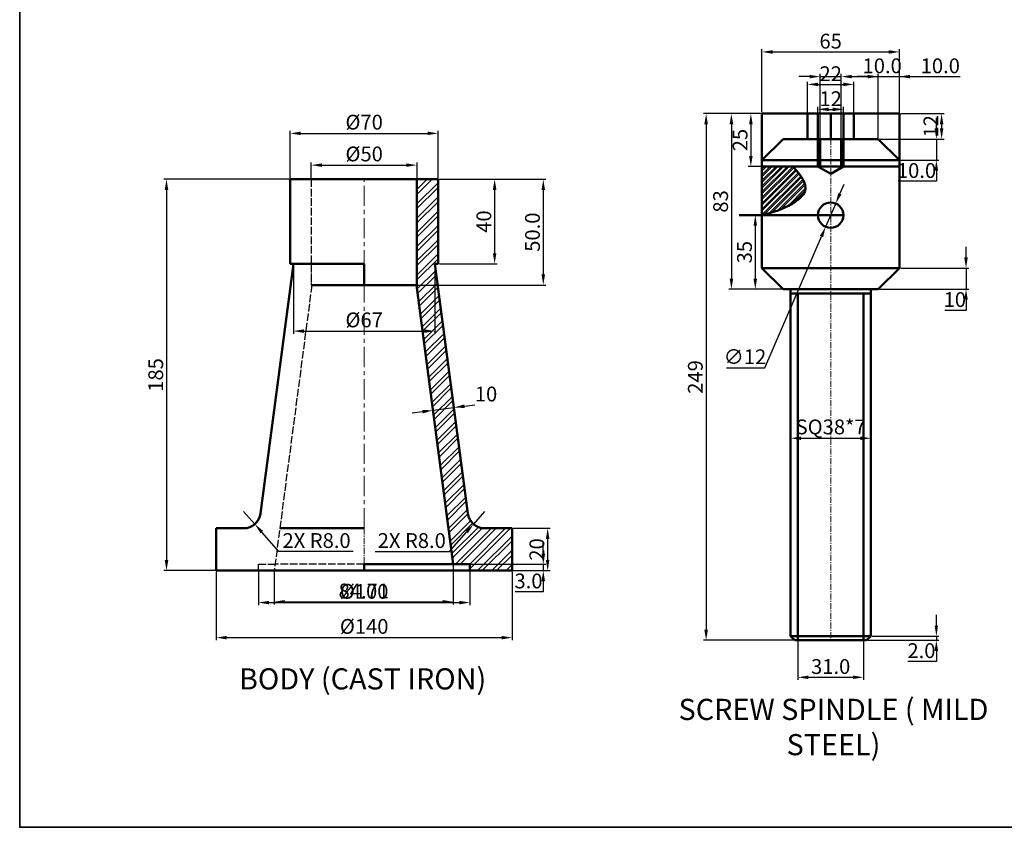
# Model space of a CAD drawing. Units: millimetres. Extents: x 4274 to 5106, y 2129 to 2785.
# Tile 1 of 4: x 4274 to 4740, y 2140 to 2522. Entities that reach past the tile are written whole.
import ezdxf

# ---------------------------------------------------------------- set-up
doc = ezdxf.new("R2010")
doc.units = ezdxf.units.MM
doc.header["$LTSCALE"] = 0.3
doc.linetypes.add('ACAD_ISO02W100', pattern=[15, 12, -3])
doc.linetypes.add('CENTER', pattern=[50.8, 31.75, -6.35, 6.35, -6.35])
for name, color, linetype, lineweight in [('M-CNTR', 1, 'CENTER', 18), ('M-DIMS', 2, 'Continuous', 25), ('M-HATC', 8, 'Continuous', 18), ('M-HIDN', 8, 'ACAD_ISO02W100', 25), ('M-OUTL', 7, 'Continuous', 50), ('M-TEXT', 3, 'Continuous', 25), ('M-TTLB', 7, 'Continuous', 35)]:
    doc.layers.add(name, color=color, linetype=linetype, lineweight=lineweight)
doc.styles.get("Standard").update_dxf_attribs({"font": 'arial.ttf'})
doc.dimstyles.new('ISO-25', dxfattribs={"dimtxt": 7, "dimasz": 5, "dimexe": 1.25, "dimexo": 0.625, "dimtad": 1, "dimtoh": 1, "dimtxsty": 'Standard', "dimcen": 2.5, "dimadec": 0, "dimazin": 0, "dimtfac": 1, "dimtmove": 0, "dimatfit": 3, "dimfxl": 1, "dimarcsym": 0})

# ---------------------------------------------------------------- blocks, each defined once
blk = doc.blocks.new('*D1')
at = {"layer": 'Defpoints', "color": 0, "ltscale": 0.3, "transparency": 16777216}
for p in [(4366.95, 2261.27), (4506.95, 2261.27), (4506.95, 2229.58)]:
    blk.add_point(p, dxfattribs=at)
at = {"layer": 'M-DIMS', "color": 0, "lineweight": -2, "ltscale": 0.3, "transparency": 16777216}
for p, q in [((4366.95, 2260.64), (4366.95, 2228.33)), ((4506.95, 2260.64), (4506.95, 2228.33)), ((4371.95, 2229.58), (4501.95, 2229.58))]:
    blk.add_line(p, q, dxfattribs=at)
at = {"layer": 'M-DIMS', "color": 0, "ltscale": 0.3, "transparency": 16777216}
for points in [[(4371.95, 2230.41), (4371.95, 2228.74), (4366.95, 2229.58)], [(4501.95, 2230.41), (4501.95, 2228.74), (4506.95, 2229.58)]]:
    blk.add_solid(points, dxfattribs=at)
at = {"layer": 'M-DIMS', "color": 0, "ltscale": 0.3, "transparency": 16777216, "insert": (4436.95, 2233.97), "char_height": 7, "attachment_point": 5}
blk.add_mtext('%%C140', dxfattribs=at)
blk = doc.blocks.new('*D2')
at = {"layer": 'Defpoints', "color": 0, "ltscale": 0.3, "transparency": 16777216}
for p in [(4386.95, 2261.27), (4486.95, 2261.27), (4486.95, 2246.14)]:
    blk.add_point(p, dxfattribs=at)
at = {"layer": 'M-DIMS', "color": 0, "lineweight": -2, "ltscale": 0.3, "transparency": 16777216}
for p, q in [((4386.95, 2260.64), (4386.95, 2244.89)), ((4486.95, 2260.64), (4486.95, 2244.89)), ((4391.95, 2246.14), (4481.95, 2246.14))]:
    blk.add_line(p, q, dxfattribs=at)
at = {"layer": 'M-DIMS', "color": 0, "ltscale": 0.3, "transparency": 16777216}
for points in [[(4391.95, 2246.98), (4391.95, 2245.31), (4386.95, 2246.14)], [(4481.95, 2246.98), (4481.95, 2245.31), (4486.95, 2246.14)]]:
    blk.add_solid(points, dxfattribs=at)
at = {"layer": 'M-DIMS', "color": 0, "ltscale": 0.3, "transparency": 16777216, "insert": (4436.95, 2250.54), "char_height": 7, "attachment_point": 5}
blk.add_mtext('%%C100', dxfattribs=at)
blk = doc.blocks.new('*D3')
at = {"layer": 'Defpoints', "color": 0, "ltscale": 0.3, "transparency": 16777216}
for p in [(4506.95, 2281.27), (4506.95, 2261.27), (4523.77, 2261.27)]:
    blk.add_point(p, dxfattribs=at)
at = {"layer": 'M-DIMS', "color": 0, "lineweight": -2, "ltscale": 0.3, "transparency": 16777216}
for p, q in [((4507.57, 2281.27), (4525.02, 2281.27)), ((4523.77, 2276.27), (4523.77, 2266.27)), ((4507.57, 2261.27), (4525.02, 2261.27))]:
    blk.add_line(p, q, dxfattribs=at)
at = {"layer": 'M-DIMS', "color": 0, "ltscale": 0.3, "transparency": 16777216}
for points in [[(4522.93, 2276.27), (4524.6, 2276.27), (4523.77, 2281.27)], [(4522.93, 2266.27), (4524.6, 2266.27), (4523.77, 2261.27)]]:
    blk.add_solid(points, dxfattribs=at)
at = {"layer": 'M-DIMS', "color": 0, "ltscale": 0.3, "transparency": 16777216, "insert": (4519.57, 2271.27), "char_height": 7, "attachment_point": 5, "rotation": 90}
blk.add_mtext('20', dxfattribs=at)
blk = doc.blocks.new('*D4')
at = {"layer": 'Defpoints', "color": 0, "ltscale": 0.3, "transparency": 16777216}
for p in [(4436.95, 2446.27), (4343.43, 2261.27), (4436.95, 2261.27)]:
    blk.add_point(p, dxfattribs=at)
at = {"layer": 'M-DIMS', "color": 0, "lineweight": -2, "ltscale": 0.3, "transparency": 16777216}
for p, q in [((4436.32, 2446.27), (4342.18, 2446.27)), ((4343.43, 2441.27), (4343.43, 2266.27)), ((4436.32, 2261.27), (4342.18, 2261.27))]:
    blk.add_line(p, q, dxfattribs=at)
at = {"layer": 'M-DIMS', "color": 0, "ltscale": 0.3, "transparency": 16777216}
for points in [[(4342.6, 2441.27), (4344.27, 2441.27), (4343.43, 2446.27)], [(4342.6, 2266.27), (4344.27, 2266.27), (4343.43, 2261.27)]]:
    blk.add_solid(points, dxfattribs=at)
at = {"layer": 'M-DIMS', "color": 0, "ltscale": 0.3, "transparency": 16777216, "insert": (4339.23, 2353.77), "char_height": 7, "attachment_point": 5, "rotation": 90}
blk.add_mtext('185', dxfattribs=at)
blk = doc.blocks.new('*D5')
at = {"layer": 'Defpoints', "color": 0, "ltscale": 0.3, "transparency": 16777216}
for p in [(4471.95, 2446.27), (4471.95, 2406.27), (4498.68, 2406.27)]:
    blk.add_point(p, dxfattribs=at)
at = {"layer": 'M-DIMS', "color": 0, "lineweight": -2, "ltscale": 0.3, "transparency": 16777216}
for p, q in [((4472.57, 2446.27), (4499.93, 2446.27)), ((4498.68, 2441.27), (4498.68, 2411.27)), ((4472.57, 2406.27), (4499.93, 2406.27))]:
    blk.add_line(p, q, dxfattribs=at)
at = {"layer": 'M-DIMS', "color": 0, "ltscale": 0.3, "transparency": 16777216}
for points in [[(4497.85, 2441.27), (4499.52, 2441.27), (4498.68, 2446.27)], [(4497.85, 2411.27), (4499.52, 2411.27), (4498.68, 2406.27)]]:
    blk.add_solid(points, dxfattribs=at)
at = {"layer": 'M-DIMS', "color": 0, "ltscale": 0.3, "transparency": 16777216, "insert": (4494.48, 2426.27), "char_height": 7, "attachment_point": 5, "rotation": 90}
blk.add_mtext('40', dxfattribs=at)
blk = doc.blocks.new('*D6')
at = {"layer": 'Defpoints', "color": 0, "ltscale": 0.3, "transparency": 16777216}
for p in [(4471.95, 2467.97), (4401.95, 2446.27), (4471.95, 2446.27)]:
    blk.add_point(p, dxfattribs=at)
at = {"layer": 'M-DIMS', "color": 0, "lineweight": -2, "ltscale": 0.3, "transparency": 16777216}
for p, q in [((4401.95, 2446.89), (4401.95, 2469.22)), ((4471.95, 2446.89), (4471.95, 2469.22)), ((4406.95, 2467.97), (4466.95, 2467.97))]:
    blk.add_line(p, q, dxfattribs=at)
at = {"layer": 'M-DIMS', "color": 0, "ltscale": 0.3, "transparency": 16777216}
for points in [[(4406.95, 2468.81), (4406.95, 2467.14), (4401.95, 2467.97)], [(4466.95, 2468.81), (4466.95, 2467.14), (4471.95, 2467.97)]]:
    blk.add_solid(points, dxfattribs=at)
at = {"layer": 'M-DIMS', "color": 0, "ltscale": 0.3, "transparency": 16777216, "insert": (4436.95, 2472.37), "char_height": 7, "attachment_point": 5}
blk.add_mtext('%%C70', dxfattribs=at)
blk = doc.blocks.new('*D7')
at = {"layer": 'Defpoints', "color": 0, "ltscale": 0.3, "transparency": 16777216}
for p in [(4461.95, 2452.96), (4411.95, 2446.27), (4461.95, 2446.27)]:
    blk.add_point(p, dxfattribs=at)
at = {"layer": 'M-DIMS', "color": 0, "lineweight": -2, "ltscale": 0.3, "transparency": 16777216}
for p, q in [((4411.95, 2446.89), (4411.95, 2454.21)), ((4416.95, 2452.96), (4456.95, 2452.96)), ((4461.95, 2446.89), (4461.95, 2454.21))]:
    blk.add_line(p, q, dxfattribs=at)
at = {"layer": 'M-DIMS', "color": 0, "ltscale": 0.3, "transparency": 16777216}
for points in [[(4416.95, 2453.79), (4416.95, 2452.13), (4411.95, 2452.96)], [(4456.95, 2453.79), (4456.95, 2452.13), (4461.95, 2452.96)]]:
    blk.add_solid(points, dxfattribs=at)
at = {"layer": 'M-DIMS', "color": 0, "ltscale": 0.3, "transparency": 16777216, "insert": (4436.95, 2457.35), "char_height": 7, "attachment_point": 5}
blk.add_mtext('%%C50', dxfattribs=at)
blk = doc.blocks.new('*D8')
at = {"layer": 'Defpoints', "color": 0, "ltscale": 0.3, "transparency": 16777216}
for p in [(4403.45, 2406.27), (4470.45, 2406.27), (4470.45, 2374.49)]:
    blk.add_point(p, dxfattribs=at)
at = {"layer": 'M-DIMS', "color": 0, "lineweight": -2, "ltscale": 0.3, "transparency": 16777216}
for p, q in [((4403.45, 2405.64), (4403.45, 2373.24)), ((4470.45, 2405.64), (4470.45, 2373.24)), ((4408.45, 2374.49), (4465.45, 2374.49))]:
    blk.add_line(p, q, dxfattribs=at)
at = {"layer": 'M-DIMS', "color": 0, "ltscale": 0.3, "transparency": 16777216}
for points in [[(4408.45, 2375.33), (4408.45, 2373.66), (4403.45, 2374.49)], [(4465.45, 2375.33), (4465.45, 2373.66), (4470.45, 2374.49)]]:
    blk.add_solid(points, dxfattribs=at)
at = {"layer": 'M-DIMS', "color": 0, "ltscale": 0.3, "transparency": 16777216, "insert": (4436.95, 2378.89), "char_height": 7, "attachment_point": 5}
blk.add_mtext('%%C67', dxfattribs=at)
blk = doc.blocks.new('*D9')
at = {"layer": 'Defpoints', "color": 0, "ltscale": 0.3, "transparency": 16777216}
for p in [(4469.5, 2337.04), (4479.41, 2338.34), (4479.41, 2338.34)]:
    blk.add_point(p, dxfattribs=at)
at = {"layer": 'M-DIMS', "color": 0, "lineweight": -2, "ltscale": 0.3, "transparency": 16777216}
for p, q in [((4479.33, 2338.96), (4479.25, 2339.58)), ((4484.37, 2339), (4489.33, 2339.65)), ((4464.54, 2336.38), (4459.59, 2335.73)), ((4469.42, 2337.66), (4469.34, 2338.28)), ((4469.5, 2337.04), (4479.41, 2338.34))]:
    blk.add_line(p, q, dxfattribs=at)
at = {"layer": 'M-DIMS', "color": 0, "ltscale": 0.3, "transparency": 16777216}
for points in [[(4484.26, 2339.83), (4484.48, 2338.17), (4479.41, 2338.34)], [(4464.43, 2337.21), (4464.65, 2335.56), (4469.5, 2337.04)]]:
    blk.add_solid(points, dxfattribs=at)
at = {"layer": 'M-DIMS', "color": 0, "ltscale": 0.3, "transparency": 16777216, "insert": (4494.62, 2343.85), "char_height": 7, "attachment_point": 5}
blk.add_mtext('10', dxfattribs=at)
blk = doc.blocks.new('*D42')
at = {"layer": 'Defpoints', "color": 0, "ltscale": 0.3, "transparency": 16777216}
for p in [(4663.68, 2479.33), (4651.68, 2477.31), (4663.68, 2477.31)]:
    blk.add_point(p, dxfattribs=at)
at = {"layer": 'M-DIMS', "color": 0, "lineweight": -2, "ltscale": 0.3, "transparency": 16777216}
for p, q in [((4651.68, 2477.94), (4651.68, 2480.58)), ((4656.68, 2479.33), (4658.68, 2479.33)), ((4663.68, 2477.94), (4663.68, 2480.58))]:
    blk.add_line(p, q, dxfattribs=at)
at = {"layer": 'M-DIMS', "color": 0, "ltscale": 0.3, "transparency": 16777216}
for points in [[(4656.68, 2480.17), (4656.68, 2478.5), (4651.68, 2479.33)], [(4658.68, 2480.17), (4658.68, 2478.5), (4663.68, 2479.33)]]:
    blk.add_solid(points, dxfattribs=at)
at = {"layer": 'M-DIMS', "color": 0, "ltscale": 0.3, "transparency": 16777216, "insert": (4657.68, 2483.47), "char_height": 7, "attachment_point": 5}
blk.add_mtext('12', dxfattribs=at)
blk = doc.blocks.new('*D43')
at = {"layer": 'Defpoints', "color": 0, "ltscale": 0.3, "transparency": 16777216}
for p in [(4668.68, 2491.13), (4646.68, 2477.31), (4668.68, 2477.31)]:
    blk.add_point(p, dxfattribs=at)
at = {"layer": 'M-DIMS', "color": 0, "lineweight": -2, "ltscale": 0.3, "transparency": 16777216}
for p, q in [((4646.68, 2477.94), (4646.68, 2492.38)), ((4651.68, 2491.13), (4663.68, 2491.13)), ((4668.68, 2477.94), (4668.68, 2492.38))]:
    blk.add_line(p, q, dxfattribs=at)
at = {"layer": 'M-DIMS', "color": 0, "ltscale": 0.3, "transparency": 16777216}
for points in [[(4651.68, 2491.96), (4651.68, 2490.29), (4646.68, 2491.13)], [(4663.68, 2491.96), (4663.68, 2490.29), (4668.68, 2491.13)]]:
    blk.add_solid(points, dxfattribs=at)
at = {"layer": 'M-DIMS', "color": 0, "ltscale": 0.3, "transparency": 16777216, "insert": (4657.68, 2495.27), "char_height": 7, "attachment_point": 5}
blk.add_mtext('22', dxfattribs=at)
blk = doc.blocks.new('*D44')
at = {"layer": 'Defpoints', "color": 0, "ltscale": 0.3, "transparency": 16777216}
for p in [(4690.18, 2506.47), (4625.18, 2477.31), (4690.18, 2477.31)]:
    blk.add_point(p, dxfattribs=at)
at = {"layer": 'M-DIMS', "color": 0, "lineweight": -2, "ltscale": 0.3, "transparency": 16777216}
for p, q in [((4625.18, 2477.94), (4625.18, 2507.72)), ((4630.18, 2506.47), (4685.18, 2506.47)), ((4690.18, 2477.94), (4690.18, 2507.72))]:
    blk.add_line(p, q, dxfattribs=at)
at = {"layer": 'M-DIMS', "color": 0, "ltscale": 0.3, "transparency": 16777216}
for points in [[(4630.18, 2507.3), (4630.18, 2505.64), (4625.18, 2506.47)], [(4685.18, 2507.3), (4685.18, 2505.64), (4690.18, 2506.47)]]:
    blk.add_solid(points, dxfattribs=at)
at = {"layer": 'M-DIMS', "color": 0, "ltscale": 0.3, "transparency": 16777216, "insert": (4657.68, 2510.67), "char_height": 7, "attachment_point": 5}
blk.add_mtext('65', dxfattribs=at)
blk = doc.blocks.new('*D45')
at = {"layer": 'Defpoints', "color": 0, "ltscale": 0.3, "transparency": 16777216}
for p in [(4690.18, 2477.31), (4680.18, 2465.31), (4710.16, 2465.31)]:
    blk.add_point(p, dxfattribs=at)
at = {"layer": 'M-DIMS', "color": 0, "lineweight": -2, "ltscale": 0.3, "transparency": 16777216}
for p, q in [((4690.8, 2477.31), (4711.41, 2477.31)), ((4710.16, 2472.31), (4710.16, 2470.31)), ((4680.8, 2465.31), (4711.41, 2465.31))]:
    blk.add_line(p, q, dxfattribs=at)
at = {"layer": 'M-DIMS', "color": 0, "ltscale": 0.3, "transparency": 16777216}
for points in [[(4709.33, 2472.31), (4710.99, 2472.31), (4710.16, 2477.31)], [(4709.33, 2470.31), (4710.99, 2470.31), (4710.16, 2465.31)]]:
    blk.add_solid(points, dxfattribs=at)
at = {"layer": 'M-DIMS', "color": 0, "ltscale": 0.3, "transparency": 16777216, "insert": (4706.02, 2471.31), "char_height": 7, "attachment_point": 5, "rotation": 90}
blk.add_mtext('12', dxfattribs=at)
blk = doc.blocks.new('*D46')
at = {"layer": 'Defpoints', "color": 0, "ltscale": 0.3, "transparency": 16777216}
for p in [(4690.18, 2404.31), (4680.18, 2394.31), (4721.72, 2394.31)]:
    blk.add_point(p, dxfattribs=at)
at = {"layer": 'M-DIMS', "color": 0, "lineweight": -2, "ltscale": 0.3, "transparency": 16777216}
for p, q in [((4721.72, 2409.31), (4721.72, 2414.31)), ((4690.8, 2404.31), (4722.97, 2404.31)), ((4721.72, 2404.31), (4721.72, 2394.31)), ((4680.8, 2394.31), (4722.97, 2394.31)), ((4721.72, 2389.31), (4721.72, 2384.31)), ((4721.72, 2384.31), (4711.75, 2384.31))]:
    blk.add_line(p, q, dxfattribs=at)
at = {"layer": 'M-DIMS', "color": 0, "ltscale": 0.3, "transparency": 16777216}
for points in [[(4720.88, 2409.31), (4722.55, 2409.31), (4721.72, 2404.31)], [(4720.88, 2389.31), (4722.55, 2389.31), (4721.72, 2394.31)]]:
    blk.add_solid(points, dxfattribs=at)
at = {"layer": 'M-DIMS', "color": 0, "ltscale": 0.3, "transparency": 16777216, "insert": (4716.42, 2388.51), "char_height": 7, "attachment_point": 5}
blk.add_mtext('10', dxfattribs=at)
blk = doc.blocks.new('*D47')
at = {"layer": 'Defpoints', "color": 0, "ltscale": 0.3, "transparency": 16777216}
for p in [(4625.18, 2477.31), (4598.74, 2228.31), (4640.68, 2228.31)]:
    blk.add_point(p, dxfattribs=at)
at = {"layer": 'M-DIMS', "color": 0, "lineweight": -2, "ltscale": 0.3, "transparency": 16777216}
for p, q in [((4624.55, 2477.31), (4597.49, 2477.31)), ((4598.74, 2472.31), (4598.74, 2233.31)), ((4640.05, 2228.31), (4597.49, 2228.31))]:
    blk.add_line(p, q, dxfattribs=at)
at = {"layer": 'M-DIMS', "color": 0, "ltscale": 0.3, "transparency": 16777216}
for points in [[(4597.91, 2472.31), (4599.57, 2472.31), (4598.74, 2477.31)], [(4597.91, 2233.31), (4599.57, 2233.31), (4598.74, 2228.31)]]:
    blk.add_solid(points, dxfattribs=at)
at = {"layer": 'M-DIMS', "color": 0, "ltscale": 0.3, "transparency": 16777216, "insert": (4594.54, 2352.81), "char_height": 7, "attachment_point": 5, "rotation": 90}
blk.add_mtext('249', dxfattribs=at)
blk = doc.blocks.new('*D48')
at = {"layer": 'Defpoints', "color": 0, "ltscale": 0.3, "transparency": 16777216}
for p in [(4625.18, 2477.31), (4610.71, 2394.31), (4635.18, 2394.31)]:
    blk.add_point(p, dxfattribs=at)
at = {"layer": 'M-DIMS', "color": 0, "lineweight": -2, "ltscale": 0.3, "transparency": 16777216}
for p, q in [((4624.55, 2477.31), (4609.46, 2477.31)), ((4610.71, 2472.31), (4610.71, 2399.31)), ((4634.55, 2394.31), (4609.46, 2394.31))]:
    blk.add_line(p, q, dxfattribs=at)
at = {"layer": 'M-DIMS', "color": 0, "ltscale": 0.3, "transparency": 16777216}
for points in [[(4609.88, 2472.31), (4611.55, 2472.31), (4610.71, 2477.31)], [(4609.88, 2399.31), (4611.55, 2399.31), (4610.71, 2394.31)]]:
    blk.add_solid(points, dxfattribs=at)
at = {"layer": 'M-DIMS', "color": 0, "ltscale": 0.3, "transparency": 16777216, "insert": (4606.51, 2435.81), "char_height": 7, "attachment_point": 5, "rotation": 90}
blk.add_mtext('83', dxfattribs=at)
blk = doc.blocks.new('*D49')
at = {"layer": 'Defpoints', "color": 0, "ltscale": 0.3, "transparency": 16777216}
for p in [(4625.18, 2429.31), (4622.01, 2394.31), (4635.18, 2394.31)]:
    blk.add_point(p, dxfattribs=at)
at = {"layer": 'M-DIMS', "color": 0, "lineweight": -2, "ltscale": 0.3, "transparency": 16777216}
for p, q in [((4624.55, 2429.31), (4620.76, 2429.31)), ((4622.01, 2424.31), (4622.01, 2399.31)), ((4634.55, 2394.31), (4620.76, 2394.31))]:
    blk.add_line(p, q, dxfattribs=at)
at = {"layer": 'M-DIMS', "color": 0, "ltscale": 0.3, "transparency": 16777216}
for points in [[(4621.17, 2424.31), (4622.84, 2424.31), (4622.01, 2429.31)], [(4621.17, 2399.31), (4622.84, 2399.31), (4622.01, 2394.31)]]:
    blk.add_solid(points, dxfattribs=at)
at = {"layer": 'M-DIMS', "color": 0, "ltscale": 0.3, "transparency": 16777216, "insert": (4617.81, 2411.81), "char_height": 7, "attachment_point": 5, "rotation": 90}
blk.add_mtext('35', dxfattribs=at)
blk = doc.blocks.new('*D50')
at = {"layer": 'Defpoints', "color": 0, "ltscale": 0.3, "transparency": 16777216}
for p in [(4625.18, 2477.31), (4619.92, 2452.31), (4625.18, 2452.31)]:
    blk.add_point(p, dxfattribs=at)
at = {"layer": 'M-DIMS', "color": 0, "lineweight": -2, "ltscale": 0.3, "transparency": 16777216}
for p, q in [((4624.55, 2477.31), (4618.67, 2477.31)), ((4619.92, 2472.31), (4619.92, 2457.31)), ((4624.55, 2452.31), (4618.67, 2452.31))]:
    blk.add_line(p, q, dxfattribs=at)
at = {"layer": 'M-DIMS', "color": 0, "ltscale": 0.3, "transparency": 16777216}
for points in [[(4619.09, 2472.31), (4620.75, 2472.31), (4619.92, 2477.31)], [(4619.09, 2457.31), (4620.75, 2457.31), (4619.92, 2452.31)]]:
    blk.add_solid(points, dxfattribs=at)
at = {"layer": 'M-DIMS', "color": 0, "ltscale": 0.3, "transparency": 16777216, "insert": (4615.72, 2464.81), "char_height": 7, "attachment_point": 5, "rotation": 90}
blk.add_mtext('25', dxfattribs=at)
blk = doc.blocks.new('*D51')
at = {"layer": 'Defpoints', "color": 0, "ltscale": 0.3, "transparency": 16777216}
for p in [(4676.68, 2323.83), (4638.68, 2312.31), (4676.68, 2312.31)]:
    blk.add_point(p, dxfattribs=at)
at = {"layer": 'M-DIMS', "color": 0, "lineweight": -2, "ltscale": 0.3, "transparency": 16777216}
for p, q in [((4638.68, 2312.94), (4638.68, 2325.08)), ((4676.68, 2312.94), (4676.68, 2325.08)), ((4643.68, 2323.83), (4671.68, 2323.83))]:
    blk.add_line(p, q, dxfattribs=at)
at = {"layer": 'M-DIMS', "color": 0, "ltscale": 0.3, "transparency": 16777216}
for points in [[(4643.68, 2324.66), (4643.68, 2323), (4638.68, 2323.83)], [(4671.68, 2324.66), (4671.68, 2323), (4676.68, 2323.83)]]:
    blk.add_solid(points, dxfattribs=at)
at = {"layer": 'M-DIMS', "color": 0, "ltscale": 0.3, "transparency": 16777216, "insert": (4657.68, 2328.29), "char_height": 7, "attachment_point": 5}
blk.add_mtext('SQ38*7', dxfattribs=at)
blk = doc.blocks.new('*D52')
at = {"layer": 'Defpoints', "color": 0, "ltscale": 0.3, "transparency": 16777216}
for p in [(4660.05, 2434.82), (4655.3, 2423.8)]:
    blk.add_point(p, dxfattribs=at)
at = {"layer": 'M-DIMS', "color": 0, "lineweight": -2, "ltscale": 0.3, "transparency": 16777216}
for p, q in [((4662.03, 2439.41), (4664.01, 2444.01)), ((4660.05, 2434.82), (4655.3, 2423.8)), ((4626.53, 2357.07), (4653.32, 2419.21)), ((4608.33, 2357.07), (4626.53, 2357.07))]:
    blk.add_line(p, q, dxfattribs=at)
at = {"layer": 'M-DIMS', "color": 0, "ltscale": 0.3, "transparency": 16777216}
for points in [[(4661.27, 2439.74), (4662.8, 2439.08), (4660.05, 2434.82)], [(4652.56, 2419.54), (4654.09, 2418.88), (4655.3, 2423.8)]]:
    blk.add_solid(points, dxfattribs=at)
at = {"layer": 'M-DIMS', "color": 0, "ltscale": 0.3, "transparency": 16777216, "insert": (4617.12, 2361.46), "char_height": 7, "attachment_point": 5}
blk.add_mtext('∅12', dxfattribs=at)
blk = doc.blocks.new('*D62')
at = {"layer": 'Defpoints', "color": 0, "ltscale": 0.3, "transparency": 16777216}
for p in [(4461.95, 2446.27), (4461.68, 2396.27), (4521.7, 2396.27)]:
    blk.add_point(p, dxfattribs=at)
at = {"layer": 'M-DIMS', "color": 0, "lineweight": -2, "ltscale": 0.3, "transparency": 16777216}
for p, q in [((4462.57, 2446.27), (4522.95, 2446.27)), ((4521.7, 2441.27), (4521.7, 2401.27)), ((4462.31, 2396.27), (4522.95, 2396.27))]:
    blk.add_line(p, q, dxfattribs=at)
at = {"layer": 'M-DIMS', "color": 0, "ltscale": 0.3, "transparency": 16777216}
for points in [[(4520.86, 2441.27), (4522.53, 2441.27), (4521.7, 2446.27)], [(4520.86, 2401.27), (4522.53, 2401.27), (4521.7, 2396.27)]]:
    blk.add_solid(points, dxfattribs=at)
at = {"layer": 'M-DIMS', "color": 0, "ltscale": 0.3, "transparency": 16777216, "insert": (4517.5, 2421.27), "char_height": 7, "attachment_point": 5, "rotation": 90}
blk.add_mtext('50.0', dxfattribs=at)
blk = doc.blocks.new('*D63')
at = {"layer": 'Defpoints', "color": 0, "ltscale": 0.3, "transparency": 16777216}
for p in [(4479.1, 2264.27), (4394.39, 2261.27), (4479.1, 2246.52)]:
    blk.add_point(p, dxfattribs=at)
at = {"layer": 'M-DIMS', "color": 0, "lineweight": -2, "ltscale": 0.3, "transparency": 16777216}
for p, q in [((4394.39, 2260.64), (4394.39, 2245.27)), ((4479.1, 2263.64), (4479.1, 2245.27)), ((4399.39, 2246.52), (4474.1, 2246.52))]:
    blk.add_line(p, q, dxfattribs=at)
at = {"layer": 'M-DIMS', "color": 0, "ltscale": 0.3, "transparency": 16777216}
for points in [[(4399.39, 2247.35), (4399.39, 2245.68), (4394.39, 2246.52)], [(4474.1, 2247.35), (4474.1, 2245.68), (4479.1, 2246.52)]]:
    blk.add_solid(points, dxfattribs=at)
at = {"layer": 'M-DIMS', "color": 0, "ltscale": 0.3, "transparency": 16777216, "insert": (4436.75, 2250.72), "char_height": 7, "attachment_point": 5}
blk.add_mtext('84.71', dxfattribs=at)
blk = doc.blocks.new('*D64')
at = {"layer": 'Defpoints', "color": 0, "ltscale": 0.3, "transparency": 16777216}
for p in [(4486.95, 2264.27), (4486.95, 2261.27), (4521.7, 2261.27)]:
    blk.add_point(p, dxfattribs=at)
at = {"layer": 'M-DIMS', "color": 0, "lineweight": -2, "ltscale": 0.3, "transparency": 16777216}
for p, q in [((4521.7, 2269.27), (4521.7, 2274.27)), ((4487.57, 2264.27), (4522.95, 2264.27)), ((4521.7, 2264.27), (4521.7, 2261.27)), ((4487.57, 2261.27), (4522.95, 2261.27)), ((4521.7, 2256.27), (4521.7, 2251.27)), ((4521.7, 2251.27), (4508.36, 2251.27))]:
    blk.add_line(p, q, dxfattribs=at)
at = {"layer": 'M-DIMS', "color": 0, "ltscale": 0.3, "transparency": 16777216}
for points in [[(4520.86, 2269.27), (4522.53, 2269.27), (4521.7, 2264.27)], [(4520.86, 2256.27), (4522.53, 2256.27), (4521.7, 2261.27)]]:
    blk.add_solid(points, dxfattribs=at)
at = {"layer": 'M-DIMS', "color": 0, "ltscale": 0.3, "transparency": 16777216, "insert": (4514.71, 2255.47), "char_height": 7, "attachment_point": 5}
blk.add_mtext('3.0', dxfattribs=at)
blk = doc.blocks.new('*D65')
at = {"layer": 'Defpoints', "color": 0, "ltscale": 0.3, "transparency": 16777216}
for p in [(4680.18, 2465.31), (4690.18, 2455.31), (4707.68, 2455.31)]:
    blk.add_point(p, dxfattribs=at)
at = {"layer": 'M-DIMS', "color": 0, "lineweight": -2, "ltscale": 0.3, "transparency": 16777216}
for p, q in [((4707.68, 2470.31), (4707.68, 2475.31)), ((4680.8, 2465.31), (4708.93, 2465.31)), ((4707.68, 2465.31), (4707.68, 2455.31)), ((4690.8, 2455.31), (4708.93, 2455.31)), ((4707.68, 2450.31), (4707.68, 2445.31)), ((4707.68, 2445.31), (4689.55, 2445.31))]:
    blk.add_line(p, q, dxfattribs=at)
at = {"layer": 'M-DIMS', "color": 0, "ltscale": 0.3, "transparency": 16777216}
for points in [[(4706.84, 2470.31), (4708.51, 2470.31), (4707.68, 2465.31)], [(4706.84, 2450.31), (4708.51, 2450.31), (4707.68, 2455.31)]]:
    blk.add_solid(points, dxfattribs=at)
at = {"layer": 'M-DIMS', "color": 0, "ltscale": 0.3, "transparency": 16777216, "insert": (4698.3, 2449.51), "char_height": 7, "attachment_point": 5}
blk.add_mtext('10.0', dxfattribs=at)
blk = doc.blocks.new('*D66')
at = {"layer": 'Defpoints', "color": 0, "ltscale": 0.3, "transparency": 16777216}
for p in [(4690.18, 2494.81), (4680.18, 2465.31), (4690.18, 2455.31)]:
    blk.add_point(p, dxfattribs=at)
at = {"layer": 'M-DIMS', "color": 0, "lineweight": -2, "ltscale": 0.3, "transparency": 16777216}
for p, q in [((4675.18, 2494.81), (4670.18, 2494.81)), ((4680.18, 2465.94), (4680.18, 2496.06)), ((4680.18, 2494.81), (4690.18, 2494.81)), ((4690.18, 2455.94), (4690.18, 2496.06)), ((4695.18, 2494.81), (4718.93, 2494.81))]:
    blk.add_line(p, q, dxfattribs=at)
at = {"layer": 'M-DIMS', "color": 0, "ltscale": 0.3, "transparency": 16777216}
for points in [[(4675.18, 2495.65), (4675.18, 2493.98), (4680.18, 2494.81)], [(4695.18, 2495.65), (4695.18, 2493.98), (4690.18, 2494.81)]]:
    blk.add_solid(points, dxfattribs=at)
at = {"layer": 'M-DIMS', "color": 0, "ltscale": 0.3, "transparency": 16777216, "insert": (4709.55, 2499.01), "char_height": 7, "attachment_point": 5}
blk.add_mtext('10.0', dxfattribs=at)
blk = doc.blocks.new('*D67')
at = {"layer": 'Defpoints', "color": 0, "ltscale": 0.3, "transparency": 16777216}
for p in [(4662.68, 2494.81), (4652.68, 2465.31), (4662.68, 2465.31)]:
    blk.add_point(p, dxfattribs=at)
at = {"layer": 'M-DIMS', "color": 0, "lineweight": -2, "ltscale": 0.3, "transparency": 16777216}
for p, q in [((4647.68, 2494.81), (4642.68, 2494.81)), ((4652.68, 2465.94), (4652.68, 2496.06)), ((4652.68, 2494.81), (4662.68, 2494.81)), ((4662.68, 2465.94), (4662.68, 2496.06)), ((4667.68, 2494.81), (4691.43, 2494.81))]:
    blk.add_line(p, q, dxfattribs=at)
at = {"layer": 'M-DIMS', "color": 0, "ltscale": 0.3, "transparency": 16777216}
for points in [[(4647.68, 2495.65), (4647.68, 2493.98), (4652.68, 2494.81)], [(4667.68, 2495.65), (4667.68, 2493.98), (4662.68, 2494.81)]]:
    blk.add_solid(points, dxfattribs=at)
at = {"layer": 'M-DIMS', "color": 0, "ltscale": 0.3, "transparency": 16777216, "insert": (4682.05, 2499.01), "char_height": 7, "attachment_point": 5}
blk.add_mtext('10.0', dxfattribs=at)
blk = doc.blocks.new('*D68')
at = {"layer": 'Defpoints', "color": 0, "ltscale": 0.3, "transparency": 16777216}
for p in [(4642.18, 2228.31), (4673.18, 2228.31), (4673.18, 2210.81)]:
    blk.add_point(p, dxfattribs=at)
at = {"layer": 'M-DIMS', "color": 0, "lineweight": -2, "ltscale": 0.3, "transparency": 16777216}
for p, q in [((4642.18, 2227.69), (4642.18, 2209.56)), ((4673.18, 2227.69), (4673.18, 2209.56)), ((4647.18, 2210.81), (4668.18, 2210.81))]:
    blk.add_line(p, q, dxfattribs=at)
at = {"layer": 'M-DIMS', "color": 0, "ltscale": 0.3, "transparency": 16777216}
for points in [[(4647.18, 2211.65), (4647.18, 2209.98), (4642.18, 2210.81)], [(4668.18, 2211.65), (4668.18, 2209.98), (4673.18, 2210.81)]]:
    blk.add_solid(points, dxfattribs=at)
at = {"layer": 'M-DIMS', "color": 0, "ltscale": 0.3, "transparency": 16777216, "insert": (4657.68, 2215.01), "char_height": 7, "attachment_point": 5}
blk.add_mtext('31.0', dxfattribs=at)
blk = doc.blocks.new('*D69')
at = {"layer": 'Defpoints', "color": 0, "ltscale": 0.3, "transparency": 16777216}
for p in [(4674.68, 2228.31), (4676.68, 2230.31), (4707.68, 2228.31)]:
    blk.add_point(p, dxfattribs=at)
at = {"layer": 'M-DIMS', "color": 0, "lineweight": -2, "ltscale": 0.3, "transparency": 16777216}
for p, q in [((4707.68, 2235.31), (4707.68, 2240.31)), ((4675.3, 2228.31), (4708.93, 2228.31)), ((4677.3, 2230.31), (4708.93, 2230.31)), ((4707.68, 2230.31), (4707.68, 2228.31)), ((4707.68, 2223.31), (4707.68, 2218.31)), ((4707.68, 2218.31), (4694.21, 2218.31))]:
    blk.add_line(p, q, dxfattribs=at)
at = {"layer": 'M-DIMS', "color": 0, "ltscale": 0.3, "transparency": 16777216}
for points in [[(4706.84, 2235.31), (4708.51, 2235.31), (4707.68, 2230.31)], [(4706.84, 2223.31), (4708.51, 2223.31), (4707.68, 2228.31)]]:
    blk.add_solid(points, dxfattribs=at)
at = {"layer": 'M-DIMS', "color": 0, "ltscale": 0.3, "transparency": 16777216, "insert": (4700.63, 2222.51), "char_height": 7, "attachment_point": 5}
blk.add_mtext('2.0', dxfattribs=at)
blk = doc.blocks.new('*D73')
at = {"layer": 'Defpoints', "color": 0, "ltscale": 0.3, "transparency": 16777216}
for p in [(4379.93, 2289.27), (4385.21, 2283.25)]:
    blk.add_point(p, dxfattribs=at)
at = {"layer": 'M-DIMS', "color": 0, "lineweight": -2, "ltscale": 0.3, "transparency": 16777216}
for p, q in [((4379.93, 2289.27), (4385.21, 2283.25)), ((4396.51, 2270.36), (4388.5, 2279.49)), ((4431.72, 2270.36), (4396.51, 2270.36))]:
    blk.add_line(p, q, dxfattribs=at)
at = {"layer": 'M-DIMS', "color": 0, "ltscale": 0.3, "transparency": 16777216}
blk.add_solid([(4389.13, 2280.04), (4387.88, 2278.94), (4385.21, 2283.25)], dxfattribs=at)
at = {"layer": 'M-DIMS', "color": 0, "ltscale": 0.3, "transparency": 16777216, "insert": (4414.43, 2274.56), "char_height": 7, "attachment_point": 5}
blk.add_mtext('2X R8.0', dxfattribs=at)
blk = doc.blocks.new('*D90')
at = {"layer": 'Defpoints', "color": 0, "ltscale": 0.3, "transparency": 16777216}
for p in [(4493.96, 2289.27), (4488.69, 2283.25)]:
    blk.add_point(p, dxfattribs=at)
at = {"layer": 'M-DIMS', "color": 0, "lineweight": -2, "ltscale": 0.3, "transparency": 16777216}
for p, q in [((4493.96, 2289.27), (4488.69, 2283.25)), ((4477.38, 2270.36), (4485.39, 2279.49)), ((4442.18, 2270.36), (4477.38, 2270.36))]:
    blk.add_line(p, q, dxfattribs=at)
at = {"layer": 'M-DIMS', "color": 0, "ltscale": 0.3, "transparency": 16777216}
blk.add_solid([(4484.76, 2280.04), (4486.02, 2278.94), (4488.69, 2283.25)], dxfattribs=at)
at = {"layer": 'M-DIMS', "color": 0, "ltscale": 0.3, "transparency": 16777216, "insert": (4459.47, 2274.56), "char_height": 7, "attachment_point": 5}
blk.add_mtext('2X R8.0', dxfattribs=at)

msp = doc.modelspace()

# ---------------------------------------------------------------- hatches: boundary and pattern name
at = {"layer": 'M-HATC', "ltscale": 0.3}
h = msp.add_hatch(dxfattribs=at)
h.set_pattern_fill('ANSI32', color=256, scale=0.2)
edge = h.paths.add_edge_path()
edge.add_spline(control_points=[(4625.1771, 2429.3126), (4629.9847, 2430.5861), (4637.425, 2432.5569), (4648.8242, 2441.5779), (4643.3248, 2448.2716), (4640.0048, 2452.3126)], knot_values=[0, 0, 0, 0, 15.40346786, 23.83813562, 36.68724277, 36.68724277, 36.68724277, 36.68724277], degree=3, periodic=0)
edge.add_line((4640.0048, 2452.3126), (4625.1771, 2452.3126))
edge.add_line((4625.1771, 2452.3126), (4625.1771, 2429.3126))
h = msp.add_hatch(dxfattribs=at)
h.set_pattern_fill('ANSI32', color=256, scale=0.5)
h.paths.add_polyline_path([(4470.4476, 2406.2681), (4471.9476, 2406.2681), (4471.9476, 2446.2681), (4461.9476, 2446.2681), (4461.9476, 2396.2681), (4461.6809, 2396.2681), (4479.1049, 2264.2681), (4486.9476, 2264.2681), (4486.9476, 2261.2681), (4506.9476, 2261.2681), (4506.9476, 2281.2681), (4493.961, 2281.2681, -0.37627586), (4486.0298, 2288.2211)])

# ---------------------------------------------------------------- linework, layer by layer
at = {"layer": 'M-CNTR', "ltscale": 0.3}
for p, q in [((4657.6771, 2465.3126), (4657.6771, 2228.3126)), ((4436.9476, 2281.2681), (4436.9476, 2264.2681))]:
    msp.add_line(p, q, dxfattribs=at)
at = {"layer": 'M-CNTR'}
msp.add_line((4436.9476, 2281.2681), (4436.9476, 2446.2681), dxfattribs=at)
at = {"layer": 'M-HIDN'}
for p, q in [((4411.9476, 2446.2681), (4411.9476, 2396.2681)), ((4411.9476, 2406.2681), (4411.9476, 2396.2681)), ((4412.2143, 2396.2681), (4394.3943, 2261.2681)), ((4386.9476, 2261.2681), (4386.9476, 2264.2681)), ((4386.9476, 2264.2681), (4394.7903, 2264.2681)), ((4436.9476, 2264.2681), (4394.7903, 2264.2681))]:
    msp.add_line(p, q, dxfattribs=at)
at = {"layer": 'M-OUTL', "ltscale": 0.3}
for p, q in [((4625.1771, 2477.3126), (4625.1771, 2404.3126)), ((4625.1771, 2477.3126), (4690.1771, 2477.3126)), ((4646.6771, 2477.3126), (4646.6771, 2465.3126)), ((4651.6771, 2477.3126), (4651.6771, 2452.3126)), ((4657.6771, 2477.3126), (4657.6771, 2465.3126)), ((4657.6771, 2477.3126), (4657.6771, 2465.3126)), ((4663.6771, 2477.3126), (4663.6771, 2452.3126)), ((4663.6771, 2477.3126), (4663.6771, 2452.3126)), ((4668.6771, 2477.3126), (4668.6771, 2465.3126)), ((4690.1771, 2477.3126), (4690.1771, 2404.3126)), ((4635.1771, 2465.3126), (4625.1771, 2455.3126)), ((4635.1771, 2465.3126), (4680.1771, 2465.3126)), ((4652.6771, 2465.3126), (4652.6771, 2451.7349)), ((4662.6771, 2465.3126), (4662.6771, 2451.7349)), ((4680.1771, 2465.3126), (4690.1771, 2455.3126)), ((4625.1771, 2455.3126), (4690.1771, 2455.3126)), ((4625.1771, 2452.3126), (4690.1771, 2452.3126)), ((4651.6771, 2452.3126), (4657.6771, 2448.8465)), ((4657.6771, 2448.8465), (4663.6771, 2452.3126)), ((4614.4295, 2429.3126), (4663.6771, 2429.3126)), ((4635.1771, 2394.3126), (4625.1771, 2404.3126)), ((4625.1771, 2404.3126), (4690.1771, 2404.3126)), ((4680.1771, 2394.3126), (4690.1771, 2404.3126)), ((4635.1771, 2394.3126), (4680.1771, 2394.3126)), ((4638.6771, 2394.3126), (4638.6771, 2230.3126)), ((4638.6771, 2392.3126), (4676.6771, 2392.3126)), ((4642.1771, 2392.3126), (4642.1771, 2228.3126)), ((4673.1771, 2392.3126), (4673.1771, 2228.3126)), ((4676.6771, 2394.3126), (4676.6771, 2230.3126)), ((4640.6771, 2228.3126), (4638.6771, 2230.3126)), ((4638.6771, 2230.3126), (4676.6771, 2230.3126)), ((4640.6771, 2228.3126), (4674.6771, 2228.3126)), ((4674.6771, 2228.3126), (4676.6771, 2230.3126))]:
    msp.add_line(p, q, dxfattribs=at)
at = {"layer": 'M-OUTL'}
for p, q in [((4401.9476, 2446.2681), (4471.9476, 2446.2681)), ((4401.9476, 2446.2681), (4401.9476, 2406.2681)), ((4461.9476, 2446.2681), (4461.9476, 2396.2681)), ((4471.9476, 2406.2681), (4471.9476, 2446.2681)), ((4403.4476, 2406.2681), (4387.8654, 2288.2211)), ((4401.9476, 2406.2681), (4436.9476, 2406.2681)), ((4436.9476, 2406.2681), (4436.9476, 2396.2681)), ((4470.4476, 2406.2681), (4486.0298, 2288.2211)), ((4470.4476, 2406.2681), (4471.9476, 2406.2681)), ((4411.9476, 2396.2681), (4461.9476, 2396.2681)), ((4461.6809, 2396.2681), (4479.1049, 2264.2681)), ((4366.9476, 2281.2681), (4366.9476, 2261.2681)), ((4379.9342, 2281.2681), (4366.9476, 2281.2681)), ((4436.9476, 2281.2681), (4397.0343, 2281.2681)), ((4506.9476, 2281.2681), (4493.961, 2281.2681)), ((4506.9476, 2261.2681), (4506.9476, 2281.2681)), ((4436.9476, 2261.2681), (4436.9476, 2264.2681)), ((4436.9476, 2264.2681), (4486.9476, 2264.2681)), ((4486.9476, 2264.2681), (4486.9476, 2261.2681)), ((4366.9476, 2261.2681), (4506.9476, 2261.2681))]:
    msp.add_line(p, q, dxfattribs=at)
at = {"layer": 'M-OUTL', "ltscale": 0.3}
msp.add_circle((4657.6771, 2429.3126), 6, dxfattribs=at)
at = {"layer": 'M-OUTL'}
for centre, start, end in [((4379.9342, 2289.2681), 270, 352.48043), ((4493.961, 2289.2681), 187.51957, 270)]:
    msp.add_arc(centre, 8, start, end, dxfattribs=at)
at = {"layer": 'M-OUTL', "ltscale": 0.3}
msp.add_open_spline([(4625.1771, 2429.3126), (4629.9847, 2430.5861), (4637.425, 2432.5569), (4648.8242, 2441.5779), (4643.3248, 2448.2716), (4640.0048, 2452.3126)], degree=3, knots=[0, 0, 0, 0, 15.40346786, 23.83813562, 36.68724277, 36.68724277, 36.68724277, 36.68724277], dxfattribs=at)
at = {"layer": 'M-TTLB', "ltscale": 0.3}
msp.add_lwpolyline([(5077.4601, 2139.9092), (4273.9655, 2139.9092), (4273.9655, 2785.1666), (5077.4601, 2785.1666)], close=True, dxfattribs=at)

# ---------------------------------------------------------------- texts
at = {"layer": 'M-TEXT', "ltscale": 0.3, "char_height": 10, "attachment_point": 1}
for s, insert in [('BODY (CAST IRON)', (4377.7116, 2215.0746)), ('\\pxqc;SCREW SPINDLE ( MILD STEEL)', (4569.2494, 2200.6446))]:
    msp.add_mtext_dynamic_manual_height_columns(s, width=179.51725, gutter_width=12.5, heights=[0], dxfattribs=dict(at, insert=insert))

# ---------------------------------------------------------------- dimensions: what is measured, and where the dimension line sits
at = {"layer": 'M-DIMS', "ltscale": 0.3}
for base, p1, p2, override, picture, middle in [((4690.1771, 2506.4715), (4625.1771, 2477.3126), (4690.1771, 2477.3126), {"dimclrd": 0, "dimclre": 0, "dimclrt": 0}, '*D44', (4657.6771, 2510.6705)), ((4662.6771, 2494.8126), (4652.6771, 2465.3126), (4662.6771, 2465.3126), {"dimdec": 1, "dimlfac": 1, "dimrnd": 0, "dimzin": 0, "dimdsep": 46, "dimlunit": 2}, '*D67', (4682.0521, 2499.0116)), ((4690.1771, 2494.8126), (4680.1771, 2465.3126), (4690.1771, 2455.3126), {"dimdec": 1, "dimlfac": 1, "dimrnd": 0, "dimzin": 0, "dimdsep": 46, "dimlunit": 2}, '*D66', (4709.5521, 2499.0116)), ((4663.6771, 2479.3329), (4651.6771, 2477.3126), (4663.6771, 2477.3126), {"dimclrd": 0, "dimclre": 0, "dimclrt": 0}, '*D42', (4657.6771, 2483.4723)), ((4479.1049, 2246.5181), (4394.3943, 2261.2681), (4479.1049, 2264.2681), {"dimdec": 2, "dimlfac": 1, "dimrnd": 0, "dimzin": 0, "dimdsep": 46, "dimlunit": 2}, '*D63', (4436.7496, 2250.7171)), ((4673.1771, 2210.8126), (4642.1771, 2228.3126), (4673.1771, 2228.3126), {"dimdec": 1, "dimlfac": 1, "dimrnd": 0, "dimzin": 0, "dimdsep": 46, "dimlunit": 2}, '*D68', (4657.6771, 2215.014))]:
    dim = msp.add_linear_dim(base=base, p1=p1, p2=p2, dimstyle='ISO-25', override=override, dxfattribs=at)
    dim.commit()
    dim.dimension.update_dxf_attribs({"geometry": picture, "text_midpoint": middle})
dim = msp.add_linear_dim(base=(4668.6771, 2491.1259), p1=(4646.6771, 2477.3126), p2=(4668.6771, 2477.3126), dimstyle='ISO-25', override={"dimclrd": 0, "dimclre": 0, "dimclrt": 0}, dxfattribs=at)
dim.commit()
dim.dimension.update_dxf_attribs({"geometry": '*D43', "text_midpoint": (4657.6771, 2491.1259), "dimtype": 160})
for p1, p2, distance, picture, middle in [((4401.9476, 2446.2681), (4471.9476, 2446.2681), 21.7063, '*D6', (4436.9476, 2472.3691)), ((4411.9476, 2446.2681), (4461.9476, 2446.2681), 6.6906, '*D7', (4436.9476, 2457.3534)), ((4403.4476, 2406.2681), (4470.4476, 2406.2681), -31.7732, '*D8', (4436.9476, 2378.8896)), ((4366.9476, 2261.2681), (4506.9476, 2261.2681), -31.6915, '*D1', (4436.9476, 2233.9713)), ((4386.9476, 2261.2681), (4486.9476, 2261.2681), -15.1245, '*D2', (4436.9476, 2250.5383))]:
    dim = msp.add_aligned_dim(p1=p1, p2=p2, distance=distance, text='%%C<>', dimstyle='ISO-25', override={"dimclrd": 0, "dimclre": 0, "dimclrt": 0}, dxfattribs=at)
    dim.commit()
    dim.dimension.update_dxf_attribs({"geometry": picture, "text_midpoint": middle})
dim = msp.add_linear_dim(base=(4598.7411, 2228.3126), p1=(4625.1771, 2477.3126), p2=(4640.6771, 2228.3126), angle=90, dimstyle='ISO-25', override={"dimclrd": 0, "dimclre": 0, "dimclrt": 0}, dxfattribs=at)
dim.commit()
dim.dimension.update_dxf_attribs({"geometry": '*D47', "text_midpoint": (4598.7411, 2352.8126), "dimtype": 160})
for base, p1, p2, override, picture, middle in [((4610.7133, 2394.3126), (4625.1771, 2477.3126), (4635.1771, 2394.3126), {"dimclrd": 0, "dimclre": 0, "dimclrt": 0}, '*D48', (4606.5119, 2435.8126)), ((4619.921, 2452.3126), (4625.1771, 2477.3126), (4625.1771, 2452.3126), {"dimclrd": 0, "dimclre": 0, "dimclrt": 0}, '*D50', (4615.7219, 2464.8126)), ((4710.1603, 2465.3126), (4690.1771, 2477.3126), (4680.1771, 2465.3126), {"dimclrd": 0, "dimclre": 0, "dimclrt": 0}, '*D45', (4706.021, 2471.3126)), ((4707.6771, 2455.3126), (4680.1771, 2465.3126), (4690.1771, 2455.3126), {"dimdec": 1, "dimlfac": 1, "dimrnd": 0, "dimzin": 0, "dimdsep": 46, "dimlunit": 2}, '*D65', (4698.3021, 2449.5116)), ((4521.6976, 2396.2681), (4461.9476, 2446.2681), (4461.6809, 2396.2681), {"dimdec": 1, "dimlfac": 1, "dimrnd": 0, "dimzin": 0, "dimdsep": 46, "dimlunit": 2}, '*D62', (4517.4986, 2421.2681)), ((4622.0077, 2394.3126), (4625.1771, 2429.3126), (4635.1771, 2394.3126), {"dimclrd": 0, "dimclre": 0, "dimclrt": 0}, '*D49', (4617.8063, 2411.8126)), ((4721.7155, 2394.3126), (4690.1771, 2404.3126), (4680.1771, 2394.3126), {"dimclrd": 0, "dimclre": 0, "dimclrt": 0}, '*D46', (4716.4183, 2388.5116)), ((4521.6976, 2261.2681), (4486.9476, 2264.2681), (4486.9476, 2261.2681), {"dimdec": 1, "dimlfac": 1, "dimrnd": 0, "dimzin": 0, "dimdsep": 46, "dimlunit": 2}, '*D64', (4514.7148, 2255.4695)), ((4707.6771, 2228.3126), (4676.6771, 2230.3126), (4674.6771, 2228.3126), {"dimdec": 1, "dimlfac": 1, "dimrnd": 0, "dimzin": 0, "dimdsep": 46, "dimlunit": 2}, '*D69', (4700.6322, 2222.5116))]:
    dim = msp.add_linear_dim(base=base, p1=p1, p2=p2, angle=90, dimstyle='ISO-25', override=override, dxfattribs=at)
    dim.commit()
    dim.dimension.update_dxf_attribs({"geometry": picture, "text_midpoint": middle})
for p1, p2, distance, picture, middle in [((4436.9476, 2446.2681), (4436.9476, 2261.2681), -93.5155, '*D4', (4339.2331, 2353.7681)), ((4471.9476, 2446.2681), (4471.9476, 2406.2681), 26.7363, '*D5', (4494.4849, 2426.2681)), ((4469.4995, 2337.036), (4479.4135, 2338.3446), 0, '*D9', (4494.6247, 2343.8523)), ((4506.9476, 2281.2681), (4506.9476, 2261.2681), 16.8179, '*D3', (4519.5665, 2271.2681))]:
    dim = msp.add_aligned_dim(p1=p1, p2=p2, distance=distance, dimstyle='ISO-25', override={"dimclrd": 0, "dimclre": 0, "dimclrt": 0}, dxfattribs=at)
    dim.commit()
    dim.dimension.update_dxf_attribs({"geometry": picture, "text_midpoint": middle})
dim = msp.add_diameter_dim_2p(p1=(4660.0525, 2434.8223), p2=(4655.3017, 2423.8028), dimstyle='ISO-25', override={"dimclrd": 0, "dimclre": 0, "dimclrt": 0}, dxfattribs=at)
dim.commit()
dim.dimension.update_dxf_attribs({"geometry": '*D52', "text_midpoint": (4617.1193, 2357.0674), "dimtype": 163})
dim = msp.add_linear_dim(base=(4676.6771, 2323.829), p1=(4638.6771, 2312.3126), p2=(4676.6771, 2312.3126), text='SQ<>*7', dimstyle='ISO-25', override={"dimclrd": 0, "dimclre": 0, "dimclrt": 0}, dxfattribs=at)
dim.commit()
dim.dimension.update_dxf_attribs({"geometry": '*D51', "text_midpoint": (4657.6771, 2328.2883)})
for center, mpoint, picture, middle in [((4379.9342, 2289.2681), (4385.2078, 2283.2523), '*D73', (4414.4265, 2274.5564)), ((4493.961, 2289.2681), (4488.6873, 2283.2524), '*D90', (4459.4683, 2274.5568))]:
    dim = msp.add_radius_dim(center=center, mpoint=mpoint, text='2X <>', dimstyle='ISO-25', override={"dimdec": 1, "dimlfac": 1, "dimrnd": 0, "dimzin": 0, "dimdsep": 46, "dimlunit": 2}, dxfattribs=at)
    dim.commit()
    dim.dimension.update_dxf_attribs({"geometry": picture, "text_midpoint": middle})

doc.saveas('drawing.dxf')
